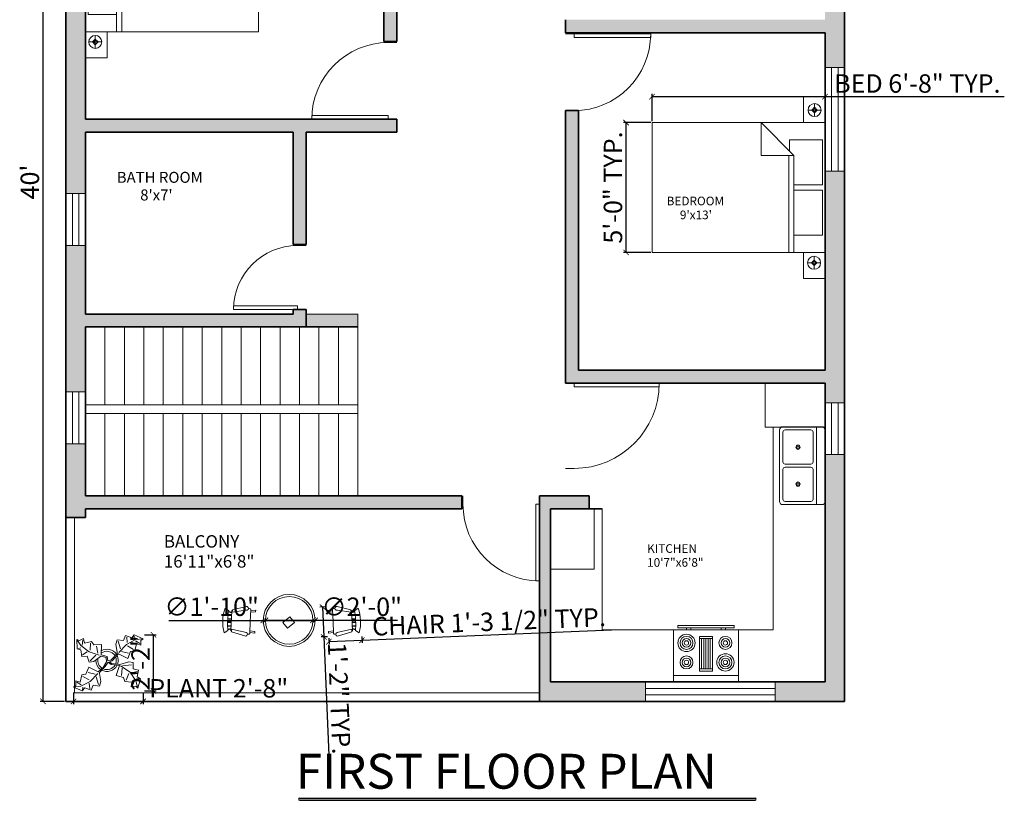
# Model space of a CAD drawing. Units: inches. Extents: x 3799 to 20199, y 1682 to 8087.
# Tile 16 of 30: x 10500 to 10956, y 7270 to 7631. Entities that reach past the tile are written whole.
import ezdxf

# ---------------------------------------------------------------- set-up
doc = ezdxf.new("R2010")
doc.units = ezdxf.units.IN
for name, color, linetype, lineweight in [('A-ANNO-DIMS', 2, 'Continuous', 18), ('A-ANNO-TITL', 7, 'Continuous', 25), ('A-AREA-IDEN', 7, 'Continuous', 18), ('A-DOOR', 3, 'Continuous', 18), ('A-EQPM', 9, 'Continuous', 18), ('A-FLOR-CASE', 32, 'Continuous', 18), ('A-FLOR-FIXT', 9, 'Continuous', 18), ('A-FLOR-RAIL', 217, 'Continuous', 18), ('A-FLOR-STRS', 41, 'Continuous', 18), ('A-FURN', 8, 'Continuous', 18), ('A-GLAZ', 152, 'Continuous', 18), ('A-WALL', 7, 'Continuous', 35), ('A-WALL-PATT', 252, 'Continuous', 13), ('L-PLNT', 94, 'Continuous', 13)]:
    doc.layers.add(name, color=color, linetype=linetype, lineweight=lineweight)
doc.styles.get("Standard").update_dxf_attribs({"font": 'arial.ttf'})
doc.dimstyles.new('ISO-25', dxfattribs={"dimtxt": 8.5, "dimasz": 2.5, "dimexe": 1.25, "dimexo": 0.625, "dimtad": 1, "dimdec": 0, "dimlunit": 3, "dimtxsty": 'Standard', "dimblk": 'ARCHTICK', "dimcen": 2.5, "dimadec": 0, "dimazin": 0, "dimtfac": 1, "dimtdec": 0, "dimtmove": 0, "dimatfit": 3, "dimfxl": 1, "dimarcsym": 0})

# ---------------------------------------------------------------- blocks, each defined once
blk = doc.blocks.new('*U170')
for p, q in [((-900, 0), (-900, 100)), ((0, 0), (0, 100))]:
    blk.add_line(p, q)
blk.add_lwpolyline([(0, 0), (0, -900), (-43.75, -900), (-43.75, 0)], close=True)
blk.add_arc((0, 0), 900, 180, 270)
blk = doc.blocks.new('*U158')
for p, q in [((0, 0), (0, -100)), ((1000, 0), (1000, -100))]:
    blk.add_line(p, q)
blk.add_lwpolyline([(0, 0), (0, 1000), (43.75, 1000), (43.75, 0)], close=True)
blk.add_arc((0, 0), 1000, 0, 90)
blk = doc.blocks.new('*U171')
for p, q in [((-750, 0), (-750, 100)), ((0, 0), (0, 100))]:
    blk.add_line(p, q)
blk.add_lwpolyline([(0, 0), (0, -750), (-43.75, -750), (-43.75, 0)], close=True)
blk.add_arc((0, 0), 750, 180, 270)
blk = doc.blocks.new('*U173')
for p, q in [((0, 0), (0, -100)), ((900, 0), (900, -100))]:
    blk.add_line(p, q)
blk.add_lwpolyline([(0, 0), (0, 900), (43.75, 900), (43.75, 0)], close=True)
blk.add_arc((0, 0), 900, 0, 90)
blk = doc.blocks.new('Bed - Queen')
for p, q in [((0, -80.00003), (0, 0)), ((0, 0), (59.99999, 0)), ((59.99999, 0), (59.99999, -80.00003)), ((7.99999, -1.2), (28.79998, -1.2)), ((7.99999, -14.4), (7.99999, -1.2)), ((28.79998, -1.2), (28.79998, -14.4)), ((31.19999, -1.2), (51.99999, -1.2)), ((31.19999, -14.4), (31.19999, -1.2)), ((51.99999, -1.2), (51.99999, -16.4)), ((0, -14.4), (44.8, -14.4)), ((44.8, -16.8), (0, -16.8)), ((59.99999, -29.6), (44.8, -14.4)), ((44.8, -14.4), (44.8, -29.6)), ((51.99999, -16.4), (46.79936, -16.4)), ((44.8, -29.6), (59.99999, -29.6)), ((59.99999, -80.00003), (0, -80.00003))]:
    blk.add_line(p, q)
blk = doc.blocks.new('Range-Oven - 30 in top')
for p, q in [((0, -3), (30, -3)), ((12, -6), (18, -6)), ((13, -20), (13, -6)), ((14, -6), (14, -20)), ((15, -20), (15, -6)), ((16, -6), (16, -20)), ((17, -20), (17, -6)), ((18, -20), (12, -20)), ((6, -24), (6, -25)), ((8, -25), (8, -24)), ((22, -25), (22, -24)), ((24, -24), (24, -25))]:
    blk.add_line(p, q)
for points in [[(0, -24), (0, 0), (30, 0), (30, -24)], [(12, -21), (12, -5), (18, -5), (18, -21)], [(2, -26), (2, -25), (28, -25), (28, -26)]]:
    blk.add_lwpolyline(points, close=True)
for centre, radius in [((6, -9), 4), ((6, -9), 3), ((6, -9), 2), ((6, -9), 1), ((24, -9), 3), ((24, -9), 2), ((24, -9), 1), ((6, -18), 3), ((6, -18), 2), ((6, -18), 1), ((24, -18), 4), ((24, -18), 3), ((24, -18), 2), ((24, -18), 1)]:
    blk.add_circle(centre, radius)
blk = doc.blocks.new('Sink-double - 36 in top')
for p, q in [((-18, -4), (18, -4)), ((-0.75, -18.5), (-0.75, -6.5)), ((0.75, -6.5), (0.75, -18.5))]:
    blk.add_line(p, q)
for points in [[(-16.5, 0), (16.5, 0)], [(-18, -19.5), (-18, -1.5)], [(18, -1.5), (18, -19.5)], [(-16.5, -18.5), (-16.5, -6.5)], [(-15.5, -5.5), (-1.75, -5.5)], [(1.75, -5.5), (15.5, -5.5)], [(16.5, -6.5), (16.5, -18.5)], [(16.5, -21), (-16.5, -21)], [(-1.75, -19.5), (-15.5, -19.5)], [(15.5, -19.5), (1.75, -19.5)]]:
    blk.add_lwpolyline(points)
for centre, radius in [((-8.5, -12.5), 1), ((-8.5, -12.5), 0.5), ((8.5, -12.5), 1), ((8.5, -12.5), 0.5)]:
    blk.add_circle(centre, radius)
for centre, radius, start, end in [((-16.5, -1.5), 1.5, 90, 180), ((16.5, -1.5), 1.5, 0, 90), ((-15.5, -6.5), 1, 90, 180), ((-1.75, -6.5), 1, 0, 90), ((1.75, -6.5), 1, 90, 180), ((15.5, -6.5), 1, 0, 90), ((-16.5, -19.5), 1.5, 180, 270), ((-15.5, -18.5), 1, 180, 270), ((-1.75, -18.5), 1, 270, 0), ((1.75, -18.5), 1, 180, 270), ((15.5, -18.5), 1, 270, 0), ((16.5, -19.5), 1.5, 270, 0)]:
    blk.add_arc(centre, radius, start, end)
blk = doc.blocks.new('Chair - Rocking')
for p, q in [((-9, -7.5), (-12, -18.49999)), ((-8, -4.5), (-10, -1.5)), ((-7, -7.5), (-9, -7.5)), ((-9, -18.49999), (-7, -7.5)), ((-8.23428, -6.99939), (-8.3093, -7.47958)), ((-8.23041, -7), (8.23915, -7)), ((-7.5, -4.5), (-7, -7)), ((-6.5, -7), (-7.02225, -4.43)), ((-4.5, -7), (-4.96674, -4.19951)), ((-4, -7), (-4.40532, -4.16272)), ((-1.5, -4.05012), (-1.5, -7)), ((-1, -7), (-1, -4.05012)), ((1, -7), (1, -4.04655)), ((1.5, -4.05012), (1.5, -7)), ((4, -7), (4.40187, -4.18694)), ((4.5, -7), (4.96761, -4.19437)), ((6.5, -7), (7, -4.4057)), ((7.5, -4.5), (7, -7)), ((7, -7.5), (9, -7.5)), ((9, -18.49999), (7, -7.5)), ((8, -4.5), (10, -1.5)), ((8.31071, -7.48854), (8.23449, -7.00073)), ((9, -7.5), (12, -18.49999)), ((-10.36644, -20.64523), (-10.5, -21.49999)), ((-9, -22.49999), (-9.5, -26.49999)), ((0, -22.49999), (-9.5, -22.49999)), ((-8, -26.49999), (-7.5, -22.49999)), ((0, -22.49999), (9.5, -22.49999)), ((8, -26.49999), (7.5, -22.49999)), ((9, -22.49999), (9.5, -26.49999)), ((10.5, -21.49999), (10.3575, -20.58798)), ((-9.5, -26.49999), (-8, -26.49999)), ((9.5, -26.49999), (8, -26.49999))]:
    blk.add_line(p, q)
for centre, radius, start, end in [((0, -34.08333), 34.08333, 72.93847, 107.0615), ((0, -68.25004), 64.25, 93.92211, 97.15267), ((0, -68.25004), 64.25, 82.84733, 93.92211), ((-10.5, -18.99999), 1.58114, 161.5651, 18.43495), ((-9.5, -21.49999), 1, 180, 270), ((10.5, -18.99999), 1.58114, 161.5651, 18.43495), ((9.5, -21.49999), 1, 270, 0)]:
    blk.add_arc(centre, radius, start, end)
blk = doc.blocks.new('Lamp - Table')
for p, q in [((-1, 0), (-7, 0)), ((0, 3), (-3, 0)), ((-3, 0), (0, -3)), ((0, 7), (0, 1)), ((3, 0), (0, 3)), ((0, -3), (3, 0)), ((1, 0), (7, 0)), ((0, -1), (0, -7))]:
    blk.add_line(p, q)
for radius in [7, 1]:
    blk.add_circle((0, 0), radius)
blk = doc.blocks.new('Plant - Rubber or Philodendron')
for p, q in [((-16.2005, 11.4774), (-13.9899, 8.1064)), ((-16.2005, 11.4774), (-14.8639, 10.7964)), ((-16.0159, 6.3329), (-16.2005, 11.4774)), ((-14.8639, 10.7964), (-12.6195, 11.8975)), ((-13.3174, 8.325), (-13.0735, 11.0065)), ((-12.6195, 11.8975), (-12.1909, 9.4345)), ((4.6914, 8.8812), (5.3859, 11.2828)), ((5.3859, 11.2828), (8.8871, 10.7908)), ((8.8871, 10.7908), (9.9809, 13.4933)), ((9.9809, 13.4933), (13.3837, 12.301)), ((15.3859, 11.3055), (10.3916, 8.7942)), ((10.5828, 12.6946), (10.8893, 9.7953)), ((13.3837, 12.301), (14.68, 13.9039)), ((14.5816, 13.2037), (14.3848, 11.8033)), ((14.68, 13.9039), (19.3848, 11.8146)), ((15.2875, 10.6053), (17.5907, 9.2105)), ((19.3848, 11.8146), (15.3859, 11.3055)), ((19.3848, 11.8146), (18.1868, 10.9119)), ((18.1868, 10.9119), (18.1925, 8.4119)), ((-14.0069, 5.8704), (-16.0159, 6.3329)), ((-15.3434, 6.5514), (-13.9984, 6.9884)), ((-13.5868, 2.2894), (-14.0069, 5.8704)), ((-13.9899, 8.1064), (-9.5434, 4.7185)), ((-12.1909, 9.4345), (-8.3829, 10.3)), ((-8.8369, 9.409), (-9.0894, 5.6095)), ((-8.3829, 10.3), (-7.0549, 8.501)), ((-7.0549, 8.501), (-3.0284, 8.6941)), ((-4.8529, 4.012), (-5.7184, 7.82)), ((-3.0284, 8.6941), (-3.0709, 3.1041)), ((4.6914, 8.8812), (5.5014, 4.4831)), ((5.9878, 10.4842), (7.1971, 6.3869)), ((10.3916, 8.7942), (6.2847, 4.4028)), ((14.2977, 6.1031), (10.9934, 7.9956)), ((14.8995, 5.3044), (12.7005, 4.8994)), ((15.7909, 9.1065), (14.8995, 5.3044)), ((18.1925, 8.4119), (15.7909, 9.1065)), ((-10.6784, 2.491), (-13.5868, 2.2894)), ((-13.1329, 3.1804), (-10.6614, 4.727)), ((-9.5858, -0.8715), (-10.6784, 2.491)), ((-9.5434, 4.7185), (-4.1917, 2.9888)), ((-9.1318, 0.0195), (-5.9793, 2.9025)), ((-7.1228, -0.443), (-3.5248, 2.2131)), ((-3.5248, 2.2131), (-3.3011, 2.4355)), ((-3.3011, 2.4355), (-0.5306, 1.7947)), ((-3.0709, 3.1041), (0.0797, 2.3163)), ((-0.5306, 1.7947), (-0.2255, -0.5527)), ((-0.5306, 1.7947), (-0.5306, 1.7947)), ((0.0797, 2.3163), (0.4866, -0.031)), ((0.4866, -0.031), (2.1141, 0.2298)), ((2.1141, 0.2298), (5.4346, 3.9146)), ((6.1032, 3.6844), (2.8262, -0.031)), ((5.4346, 3.9146), (5.5014, 4.4831)), ((11.1089, 1.1958), (6.1032, 3.6844)), ((7.7005, 4.8881), (11.5025, 3.9967)), ((12.7005, 4.8994), (11.1089, 1.1958)), ((-11.3237, -7.2629), (-9.7321, -3.5593)), ((-9.7321, -3.5593), (-4.7264, -6.0479)), ((-7.1228, -0.443), (-9.5858, -0.8715)), ((-2.019, -3.6148), (-4.7264, -6.0479)), ((-4.0579, -6.2781), (-0.9375, -3.1608)), ((-2.019, -3.6148), (-0.2255, -0.5527)), ((-0.9375, -3.1608), (0.5883, -0.8135)), ((0.5883, -0.8135), (2.2447, -2.0916)), ((2.8262, -0.031), (1.3003, -0.5527)), ((1.3003, -0.5527), (2.4193, -1.4655)), ((2.2447, -2.0916), (6.7108, -2.6626)), ((2.4193, -1.4655), (6.895, -2.1175)), ((4.943, -7.9659), (6.7108, -2.6626)), ((11.6605, -0.5413), (6.895, -2.1175)), ((12.3677, -6.1981), (7.219, -2.6772)), ((8.125, -4.0768), (7.7715, -7.9659)), ((8.3544, -2.7453), (13.1973, -2.1704)), ((11.6605, -0.5413), (14.1354, -0.8948)), ((14.1354, -0.8948), (14.1354, -4.4304)), ((14.1354, -4.4304), (16.9638, -5.1375)), ((16.9638, -5.1375), (16.2567, -8.673)), ((-14.4141, -11.4699), (-13.5228, -7.6679)), ((-13.5228, -7.6679), (-11.3237, -7.2629)), ((-12.921, -8.4665), (-9.6166, -10.359)), ((-6.3237, -7.2516), (-10.1257, -6.3602)), ((-9.0148, -11.1577), (-4.9047, -6.8122)), ((-4.611, -12.8477), (-5.8203, -8.7504)), ((-4.1246, -6.8466), (-4.0579, -6.2781)), ((-3.3146, -11.2447), (-4.1246, -6.8466)), ((8.8321, -9.0266), (4.943, -7.9659)), ((9.5392, -11.1479), (8.8321, -9.0266)), ((10.2463, -10.4408), (11.6605, -6.9053)), ((15.5496, -10.7943), (12.3677, -6.1981)), ((16.2567, -5.8446), (13.4283, -6.5517)), ((17.3174, -9.7337), (15.9032, -9.7337)), ((16.2567, -8.673), (18.0245, -9.7337)), ((18.0245, -9.7337), (16.6103, -14.6834)), ((-18.008, -14.1781), (-16.8101, -13.2754)), ((-18.008, -14.1781), (-14.0091, -13.669)), ((-13.3032, -16.2674), (-18.008, -14.1781)), ((-16.8157, -10.7754), (-14.4141, -11.4699)), ((-16.8101, -13.2754), (-16.8157, -10.7754)), ((-13.9107, -12.9688), (-16.2139, -11.574)), ((-14.0091, -13.669), (-9.0148, -11.1577)), ((-12.0069, -14.6645), (-13.3032, -16.2674)), ((-13.2048, -15.5672), (-13.008, -14.1668)), ((-8.6042, -15.8568), (-12.0069, -14.6645)), ((-9.206, -15.0581), (-9.5126, -12.1588)), ((-7.5103, -13.1543), (-8.6042, -15.8568)), ((-4.0092, -13.6463), (-7.5103, -13.1543)), ((-3.3146, -11.2447), (-4.0092, -13.6463)), ((13.4283, -11.5015), (9.5392, -11.1479)), ((13.0748, -13.9763), (13.4283, -11.5015)), ((15.5496, -13.6228), (13.0748, -13.9763)), ((14.8425, -10.7943), (13.7819, -13.2692)), ((16.6103, -14.6834), (15.5496, -10.7943)), ((16.6103, -14.6834), (15.5496, -13.6228))]:
    blk.add_line(p, q)
for centre, radius, start, end in [((0, 0), 6.1275, 34.37569, 120.1028), ((0.0308, 0.1664), 6, 178.6147, 235.1169), ((0.0308, 0.1664), 5, 168.1647, 238.6725), ((-0.0601, -0.2075), 5.2461, 33.82192, 124.9414), ((-0.2664, 0.1682), 5.2775, 338.4094, 20.03007), ((-0.098, 0.1364), 6.1288, 341.2017, 26.09184), ((-0.0234, 0.3825), 6.1492, 242.5812, 331.2714), ((-0.1102, 0.4886), 5.2883, 247.3711, 327.472)]:
    blk.add_arc(centre, radius, start, end)
blk = doc.blocks.new('_ArchTick')
at = {"color": 0, "linetype": 'ByBlock', "const_width": 0.15}
blk.add_lwpolyline([(-0.5, -0.5), (0.5, 0.5)], dxfattribs=at)
blk = doc.blocks.new('*D176')
at = {"layer": 'A-ANNO-DIMS', "color": 0, "lineweight": -2, "transparency": 16777216}
for p, q in [((10521.25, 7795.62), (10509.98, 7795.62)), ((10511.23, 7795.62), (10511.23, 7315.62)), ((10521.25, 7315.62), (10509.98, 7315.62))]:
    blk.add_line(p, q, dxfattribs=at)
at = {"layer": 'Defpoints', "color": 0, "transparency": 16777216}
for p in [(10521.87, 7795.62), (10511.23, 7315.62), (10521.87, 7315.62)]:
    blk.add_point(p, dxfattribs=at)
at = {"layer": 'A-ANNO-DIMS', "color": 0, "lineweight": -2, "transparency": 16777216, "xscale": 2.5, "yscale": 2.5, "zscale": 2.5}
for p, rotation in [((10511.23, 7795.62), 90), ((10511.23, 7315.62), 270)]:
    blk.add_blockref('_ArchTick', p, dxfattribs=dict(at, rotation=rotation))
at = {"layer": 'A-ANNO-DIMS', "color": 0, "transparency": 16777216, "insert": (10506.27, 7555.62), "char_height": 8.5, "attachment_point": 5, "rotation": 90}
blk.add_mtext("40'", dxfattribs=at)
blk = doc.blocks.new('WIN-24IN-9IN-FRAME')
for p, q in [((0, 24), (9, 24)), ((3, 0), (3, 24)), ((6, 0), (6, 24)), ((0, 0), (9, 0))]:
    blk.add_line(p, q)
blk = doc.blocks.new('WIN-48IN-9IN-FRAME')
for p, q in [((0, 0), (0, 9)), ((48, 6), (0, 6)), ((48, 0), (48, 9)), ((48, 3), (0, 3))]:
    blk.add_line(p, q)
blk = doc.blocks.new('WIN-60IN-9IN-FRAME')
for p, q in [((0, 9), (0, 0)), ((60, 6), (0, 6)), ((60, 9), (60, 0)), ((60, 3), (0, 3))]:
    blk.add_line(p, q)
blk = doc.blocks.new('*D252')
at = {"layer": 'A-ANNO-DIMS', "color": 0, "lineweight": -2, "transparency": 16777216}
for p, q in [((10792.87, 7583.69), (10792.87, 7596.31)), ((10792.87, 7595.06), (10872.87, 7595.06)), ((10872.87, 7583.69), (10872.87, 7596.31)), ((10872.87, 7595.06), (10955.77, 7595.06))]:
    blk.add_line(p, q, dxfattribs=at)
at = {"layer": 'Defpoints', "color": 0, "transparency": 16777216}
for p in [(10872.87, 7595.06), (10792.87, 7583.06), (10872.87, 7583.06)]:
    blk.add_point(p, dxfattribs=at)
at = {"layer": 'A-ANNO-DIMS', "color": 0, "lineweight": -2, "transparency": 16777216, "xscale": 2.5, "yscale": 2.5, "zscale": 2.5, "rotation": 180}
blk.add_blockref('_ArchTick', (10792.87, 7595.06), dxfattribs=at)
at = {"layer": 'A-ANNO-DIMS', "color": 0, "lineweight": -2, "transparency": 16777216, "xscale": 2.5, "yscale": 2.5, "zscale": 2.5}
blk.add_blockref('_ArchTick', (10872.87, 7595.06), dxfattribs=at)
at = {"layer": 'A-ANNO-DIMS', "color": 0, "transparency": 16777216, "insert": (10915.57, 7600.03), "char_height": 8.5, "attachment_point": 5}
blk.add_mtext('BED 6\'-8" TYP.', dxfattribs=at)
blk = doc.blocks.new('*D253')
at = {"layer": 'A-ANNO-DIMS', "color": 0, "lineweight": -2, "transparency": 16777216}
for p, q in [((10792.25, 7583.06), (10779.62, 7583.06)), ((10780.87, 7523.06), (10780.87, 7583.06)), ((10792.25, 7523.06), (10779.62, 7523.06))]:
    blk.add_line(p, q, dxfattribs=at)
at = {"layer": 'Defpoints', "color": 0, "transparency": 16777216}
for p in [(10780.87, 7583.06), (10792.87, 7583.06), (10792.87, 7523.06)]:
    blk.add_point(p, dxfattribs=at)
at = {"layer": 'A-ANNO-DIMS', "color": 0, "lineweight": -2, "transparency": 16777216, "xscale": 2.5, "yscale": 2.5, "zscale": 2.5}
for p, rotation in [((10780.87, 7583.06), 90), ((10780.87, 7523.06), 270)]:
    blk.add_blockref('_ArchTick', p, dxfattribs=dict(at, rotation=rotation))
at = {"layer": 'A-ANNO-DIMS', "color": 0, "transparency": 16777216, "insert": (10775.91, 7553.06), "char_height": 8.5, "attachment_point": 5, "rotation": 90}
blk.add_mtext('5\'-0" TYP.', dxfattribs=at)
blk = doc.blocks.new('*D318')
at = {"layer": 'A-ANNO-DIMS', "color": 0, "lineweight": -2, "transparency": 16777216}
for p, q in [((10658.76, 7343.85), (10774.17, 7348.63)), ((10643.4, 7344.88), (10643.52, 7341.97)), ((10658.69, 7345.52), (10658.81, 7342.6)), ((10643.47, 7343.22), (10658.76, 7343.85))]:
    blk.add_line(p, q, dxfattribs=at)
at = {"layer": 'Defpoints', "color": 0, "transparency": 16777216}
for p in [(10643.38, 7345.51), (10658.66, 7346.14), (10658.76, 7343.85)]:
    blk.add_point(p, dxfattribs=at)
at = {"layer": 'A-ANNO-DIMS', "color": 0, "lineweight": -2, "transparency": 16777216, "xscale": 2.5, "yscale": 2.5, "zscale": 2.5}
for p, rotation in [((10643.47, 7343.22), 182.3732176474188), ((10658.76, 7343.85), 2.373217647418867)]:
    blk.add_blockref('_ArchTick', p, dxfattribs=dict(at, rotation=rotation))
at = {"layer": 'A-ANNO-DIMS', "color": 0, "transparency": 16777216, "insert": (10717.51, 7351.31), "char_height": 8.5, "attachment_point": 5, "rotation": 2.3732}
blk.add_mtext('CHAIR 1\'-3 1/2" TYP.', dxfattribs=at)
blk = doc.blocks.new('*D319')
at = {"layer": 'A-ANNO-DIMS', "color": 0, "lineweight": -2, "transparency": 16777216}
for p, q in [((10642.18, 7359.32), (10639.26, 7359.2)), ((10640.51, 7359.25), (10641.08, 7345.41)), ((10642.75, 7345.48), (10639.84, 7345.36)), ((10641.08, 7345.41), (10643.35, 7290.7))]:
    blk.add_line(p, q, dxfattribs=at)
at = {"layer": 'Defpoints', "color": 0, "transparency": 16777216}
for p in [(10642.8, 7359.34), (10641.08, 7345.41), (10643.38, 7345.51)]:
    blk.add_point(p, dxfattribs=at)
at = {"layer": 'A-ANNO-DIMS', "color": 0, "lineweight": -2, "transparency": 16777216, "xscale": 2.5, "yscale": 2.5, "zscale": 2.5}
for p, rotation in [((10640.51, 7359.25), 92.37321764741522), ((10641.08, 7345.41), 272.3732176474152)]:
    blk.add_blockref('_ArchTick', p, dxfattribs=dict(at, rotation=rotation))
at = {"layer": 'A-ANNO-DIMS', "color": 0, "transparency": 16777216, "insert": (10647.16, 7317.01), "char_height": 8.5, "attachment_point": 5, "rotation": 272.3732}
blk.add_mtext('1\'-2" TYP.', dxfattribs=at)
blk = doc.blocks.new('*D352')
at = {"layer": 'A-ANNO-DIMS', "color": 0, "lineweight": -2, "transparency": 16777216}
for p, q in [((10525.36, 7319.78), (10525.36, 7314.33)), ((10557.53, 7319.78), (10557.53, 7314.33)), ((10525.36, 7315.58), (10557.53, 7315.58)), ((10557.53, 7315.58), (10625.02, 7315.58))]:
    blk.add_line(p, q, dxfattribs=at)
at = {"layer": 'Defpoints', "color": 0, "transparency": 16777216}
for p in [(10525.36, 7320.41), (10557.53, 7320.41), (10557.53, 7315.58)]:
    blk.add_point(p, dxfattribs=at)
at = {"layer": 'A-ANNO-DIMS', "color": 0, "lineweight": -2, "transparency": 16777216, "xscale": 2.5, "yscale": 2.5, "zscale": 2.5, "rotation": 180}
blk.add_blockref('_ArchTick', (10525.36, 7315.58), dxfattribs=at)
at = {"layer": 'A-ANNO-DIMS', "color": 0, "lineweight": -2, "transparency": 16777216, "xscale": 2.5, "yscale": 2.5, "zscale": 2.5}
blk.add_blockref('_ArchTick', (10557.53, 7315.58), dxfattribs=at)
at = {"layer": 'A-ANNO-DIMS', "color": 0, "transparency": 16777216, "insert": (10592.52, 7320.55), "char_height": 8.5, "attachment_point": 5}
blk.add_mtext('PLANT 2\'-8"', dxfattribs=at)
blk = doc.blocks.new('*D353')
at = {"layer": 'A-ANNO-DIMS', "color": 0, "lineweight": -2, "transparency": 16777216}
for p, q in [((10558.15, 7346.36), (10563.6, 7346.36)), ((10562.35, 7320.41), (10562.35, 7346.36)), ((10558.15, 7320.41), (10563.6, 7320.41))]:
    blk.add_line(p, q, dxfattribs=at)
at = {"layer": 'Defpoints', "color": 0, "transparency": 16777216}
for p in [(10557.53, 7346.36), (10562.35, 7346.36), (10557.53, 7320.41)]:
    blk.add_point(p, dxfattribs=at)
at = {"layer": 'A-ANNO-DIMS', "color": 0, "lineweight": -2, "transparency": 16777216, "xscale": 2.5, "yscale": 2.5, "zscale": 2.5}
for p, rotation in [((10562.35, 7346.36), 90), ((10562.35, 7320.41), 270)]:
    blk.add_blockref('_ArchTick', p, dxfattribs=dict(at, rotation=rotation))
at = {"layer": 'A-ANNO-DIMS', "color": 0, "transparency": 16777216, "insert": (10557.46, 7333.38), "char_height": 8.5, "attachment_point": 5, "rotation": 90}
blk.add_mtext('2\'-2"', dxfattribs=at)
blk = doc.blocks.new('*D391')
at = {"layer": 'A-ANNO-DIMS', "color": 0, "lineweight": -2, "transparency": 16777216}
for p in [(10613.1, 7353.04), (10675.19, 7353.04)]:
    blk.add_line(p, (10637.1, 7353.04), dxfattribs=at)
at = {"layer": 'Defpoints', "color": 0, "transparency": 16777216}
for p in [(10613.1, 7353.04), (10637.1, 7353.04)]:
    blk.add_point(p, dxfattribs=at)
at = {"layer": 'A-ANNO-DIMS', "color": 0, "lineweight": -2, "transparency": 16777216, "xscale": 2.5, "yscale": 2.5, "zscale": 2.5}
for p, rotation in [((10613.1, 7353.04), 359.9981044646316), ((10637.1, 7353.04), 179.9981044646316)]:
    blk.add_blockref('_ArchTick', p, dxfattribs=dict(at, rotation=rotation))
at = {"layer": 'A-ANNO-DIMS', "color": 0, "transparency": 16777216, "insert": (10658.65, 7358.24), "char_height": 8.5, "attachment_point": 5, "rotation": 359.9981}
blk.add_mtext('∅2\'-0"', dxfattribs=at)
blk = doc.blocks.new('*D392')
at = {"layer": 'A-ANNO-DIMS', "color": 0, "lineweight": -2, "transparency": 16777216}
for p in [(10569.4, 7353.04), (10636.1, 7353.04)]:
    blk.add_line(p, (10614.1, 7353.04), dxfattribs=at)
at = {"layer": 'Defpoints', "color": 0, "transparency": 16777216}
for p in [(10614.1, 7353.04), (10636.1, 7353.04)]:
    blk.add_point(p, dxfattribs=at)
at = {"layer": 'A-ANNO-DIMS', "color": 0, "lineweight": -2, "transparency": 16777216, "xscale": 2.5, "yscale": 2.5, "zscale": 2.5}
for p, rotation in [((10614.1, 7353.04), 0.0020678567677366), ((10636.1, 7353.04), 180.0020678567677)]:
    blk.add_blockref('_ArchTick', p, dxfattribs=dict(at, rotation=rotation))
at = {"layer": 'A-ANNO-DIMS', "color": 0, "transparency": 16777216, "insert": (10589.25, 7358.24), "char_height": 8.5, "attachment_point": 5, "rotation": 0.0021}
blk.add_mtext('∅1\'-10"', dxfattribs=at)

msp = doc.modelspace()

# ---------------------------------------------------------------- hatches: boundary and pattern name
at = {"layer": 'A-ANNO-TITL'}
h = msp.add_hatch(color=256, dxfattribs=at)
h.dxf.hatch_style = 1
h.paths.add_polyline_path([(10840.51, 7270.89), (10629.95, 7270.89, 1), (10629.95, 7269.89), (10840.51, 7269.89, 1)])
at = {"layer": 'A-WALL-PATT'}
h = msp.add_hatch(color=256, dxfattribs=at)
h.dxf.hatch_style = 1
h.paths.add_polyline_path([(10588.75, 7795.62), (10521.87, 7795.62), (10521.87, 7685.33), (10530.87, 7685.33), (10530.87, 7696.98), (10530.87, 7710.62), (10620.87, 7710.62), (10620.87, 7716.62), (10530.87, 7716.62), (10530.87, 7786.62), (10588.75, 7786.62)])
h.paths.add_polyline_path([(10682.68, 7795.62), (10612.75, 7795.62), (10612.75, 7786.62), (10650.87, 7786.62), (10650.87, 7716.62), (10650.87, 7710.62), (10668.87, 7710.62), (10668.87, 7620.62), (10674.87, 7620.62), (10674.87, 7710.62), (10752.87, 7710.62), (10752.87, 7666.62), (10758.87, 7666.62), (10758.87, 7756.62), (10752.87, 7756.62), (10752.87, 7716.62), (10656.87, 7716.62), (10656.87, 7786.62), (10682.68, 7786.62)])
h.paths.add_polyline_path([(10881.87, 7795.62), (10706.68, 7795.62), (10706.68, 7786.62), (10752.87, 7786.62), (10758.87, 7786.62), (10872.87, 7786.62), (10872.87, 7747.36), (10881.87, 7747.36)])
h.paths.add_polyline_path([(10881.87, 7699.36), (10872.87, 7699.36), (10872.87, 7630.62), (10752.87, 7630.62), (10752.87, 7624.62), (10872.87, 7624.62), (10872.87, 7608.58), (10881.87, 7608.58)])
h.paths.add_polyline_path([(10674.87, 7584.62), (10530.87, 7584.62), (10530.87, 7637.33), (10521.87, 7637.33), (10521.87, 7550.27), (10530.87, 7550.27), (10530.87, 7578.62), (10626.87, 7578.62), (10626.87, 7526.73), (10632.87, 7526.73), (10632.87, 7578.62), (10674.87, 7578.62)])
h.paths.add_polyline_path([(10530.87, 7488.62), (10632.87, 7488.62), (10632.87, 7496.73), (10628.93, 7496.73), (10626.87, 7496.73), (10626.87, 7494.62), (10530.87, 7494.62), (10530.87, 7526.27), (10521.87, 7526.27), (10521.87, 7458.64), (10530.87, 7458.64)])
h.paths.add_polyline_path([(10656.87, 7494.62), (10632.87, 7494.62), (10632.87, 7488.62), (10656.87, 7488.62)])
h.paths.add_polyline_path([(10530.87, 7434.64), (10521.87, 7434.64), (10521.87, 7400.54), (10530.87, 7400.54), (10530.87, 7404.62), (10704.87, 7404.62), (10704.87, 7410.62), (10530.87, 7410.62)])
h.paths.add_polyline_path([(10745.87, 7404.62), (10763.75, 7404.62), (10763.75, 7410.62), (10740.87, 7410.62), (10740.87, 7315.62), (10789.88, 7315.62), (10789.88, 7324.62), (10745.87, 7324.62)])
h.paths.add_polyline_path([(10881.87, 7429.64), (10872.87, 7429.64), (10872.87, 7408.03), (10872.87, 7324.62), (10849.88, 7324.62), (10849.88, 7315.62), (10881.87, 7315.62)])
h.paths.add_polyline_path([(10881.87, 7560.58), (10872.87, 7560.58), (10872.87, 7468.62), (10758.87, 7468.62), (10758.87, 7588.62), (10752.87, 7588.62), (10752.87, 7462.62), (10872.87, 7462.62), (10872.87, 7453.64), (10881.87, 7453.64)])

# ---------------------------------------------------------------- linework, layer by layer
at = {"layer": 'A-ANNO-TITL'}
for p, q in [((10629.95, 7270.89), (10840.51, 7270.89)), ((10629.95, 7269.89), (10840.51, 7269.89))]:
    msp.add_line(p, q, dxfattribs=at)
for centre, start, end in [((10629.95, 7270.39), 90, 270), ((10840.51, 7270.39), 270, 90)]:
    msp.add_arc(centre, 0.5, start, end, dxfattribs=at)
at = {"layer": 'A-FLOR-CASE'}
for p, q in [((10845.14, 7442.32), (10845.14, 7462.62)), ((10848.87, 7442.32), (10845.14, 7442.32)), ((10848.87, 7348.62), (10848.87, 7442.32)), ((10848.87, 7442.32), (10872.87, 7442.32)), ((10769.87, 7348.62), (10769.87, 7404.62)), ((10769.87, 7348.62), (10848.87, 7348.62))]:
    msp.add_line(p, q, dxfattribs=at)
at = {"layer": 'A-FLOR-RAIL'}
for q in [(10525.8, 7400.54), (10740.87, 7319.62)]:
    msp.add_line((10525.8, 7319.62), q, dxfattribs=at)
at = {"layer": 'A-FLOR-STRS'}
for p, q in [((10632.87, 7494.62), (10656.87, 7494.62)), ((10656.87, 7488.62), (10656.87, 7494.62)), ((10539.87, 7488.62), (10539.87, 7452.62)), ((10548.87, 7488.62), (10548.87, 7452.62)), ((10557.87, 7488.62), (10557.87, 7452.62)), ((10566.87, 7488.62), (10566.87, 7452.62)), ((10575.87, 7488.62), (10575.87, 7452.62)), ((10584.87, 7488.62), (10584.87, 7452.62)), ((10593.87, 7488.62), (10593.87, 7452.62)), ((10602.87, 7488.62), (10602.87, 7452.62)), ((10611.87, 7488.62), (10611.87, 7452.62)), ((10620.87, 7488.62), (10620.87, 7452.62)), ((10629.87, 7488.62), (10629.87, 7452.62)), ((10638.87, 7488.62), (10638.87, 7452.62)), ((10647.87, 7488.62), (10647.87, 7452.62)), ((10656.87, 7488.62), (10656.87, 7410.62)), ((10656.87, 7452.62), (10530.87, 7452.62)), ((10656.87, 7448.62), (10530.87, 7448.62)), ((10539.87, 7448.62), (10539.87, 7410.62)), ((10548.87, 7448.62), (10548.87, 7410.62)), ((10557.87, 7448.62), (10557.87, 7410.62)), ((10566.87, 7448.62), (10566.87, 7410.62)), ((10575.87, 7448.62), (10575.87, 7410.62)), ((10584.87, 7448.62), (10584.87, 7410.62)), ((10593.87, 7448.62), (10593.87, 7410.62)), ((10602.87, 7448.62), (10602.87, 7410.62)), ((10611.87, 7448.62), (10611.87, 7410.62)), ((10620.87, 7448.62), (10620.87, 7410.62)), ((10629.87, 7448.62), (10629.87, 7410.62)), ((10638.87, 7448.62), (10638.87, 7410.62)), ((10647.87, 7448.62), (10647.87, 7410.62))]:
    msp.add_line(p, q, dxfattribs=at)
at = {"layer": 'A-FURN'}
for points in [[(10530.87, 7624.98), (10540.87, 7624.98), (10540.87, 7612.98), (10530.87, 7612.98)], [(10872.87, 7583.06), (10862.87, 7583.06), (10862.87, 7595.06), (10872.87, 7595.06)], [(10872.87, 7523.06), (10862.87, 7523.06), (10862.87, 7511.06), (10872.87, 7511.06)], [(10745.87, 7404.62), (10766.06, 7404.62), (10766.06, 7376.7), (10745.87, 7376.7)], [(10622.13, 7352.05), (10625.4, 7354.75), (10627.6, 7352.09), (10624.33, 7349.4)]]:
    msp.add_lwpolyline(points, close=True, dxfattribs=at)
for radius in [12, 11]:
    msp.add_circle((10625.1, 7353.04), radius, dxfattribs=at)
at = {"layer": 'A-WALL'}
for p, q in [((10521.87, 7795.62), (10521.87, 7315.62)), ((10881.87, 7315.62), (10881.87, 7795.62)), ((10530.87, 7710.62), (10530.87, 7584.62)), ((10668.87, 7710.62), (10668.87, 7620.62)), ((10674.87, 7710.62), (10674.87, 7620.62)), ((10752.87, 7630.62), (10752.87, 7624.62)), ((10872.87, 7624.62), (10752.87, 7624.62)), ((10872.87, 7468.62), (10872.87, 7624.62)), ((10674.87, 7620.62), (10668.87, 7620.62)), ((10758.87, 7588.62), (10752.87, 7588.62)), ((10752.87, 7588.62), (10752.87, 7462.62)), ((10758.87, 7588.62), (10758.87, 7468.62)), ((10674.87, 7584.62), (10530.87, 7584.62)), ((10674.87, 7584.62), (10674.87, 7578.62)), ((10530.87, 7578.62), (10530.87, 7494.62)), ((10626.87, 7578.62), (10530.87, 7578.62)), ((10626.87, 7578.62), (10626.87, 7526.73)), ((10674.87, 7578.62), (10632.87, 7578.62)), ((10632.87, 7578.62), (10632.87, 7526.73)), ((10626.87, 7526.73), (10632.87, 7526.73)), ((10626.87, 7494.62), (10530.87, 7494.62)), ((10626.87, 7496.73), (10632.87, 7496.73)), ((10626.87, 7496.73), (10626.87, 7494.62)), ((10632.87, 7496.73), (10632.87, 7488.62)), ((10656.87, 7488.62), (10530.87, 7488.62)), ((10530.87, 7488.62), (10530.87, 7410.62)), ((10872.87, 7468.62), (10758.87, 7468.62)), ((10872.87, 7462.62), (10752.87, 7462.62)), ((10872.87, 7324.62), (10872.87, 7462.62)), ((10530.87, 7410.62), (10704.87, 7410.62)), ((10704.87, 7404.62), (10704.87, 7410.62)), ((10740.87, 7315.62), (10740.87, 7410.62)), ((10740.87, 7410.62), (10763.75, 7410.62)), ((10763.75, 7410.62), (10763.75, 7404.62)), ((10530.87, 7404.62), (10704.87, 7404.62)), ((10530.87, 7404.62), (10530.87, 7400.54)), ((10745.87, 7324.62), (10745.87, 7404.62)), ((10745.87, 7404.62), (10763.75, 7404.62)), ((10763.75, 7404.62), (10769.87, 7404.62)), ((10530.87, 7400.54), (10521.87, 7400.54)), ((10745.87, 7324.62), (10872.87, 7324.62)), ((10521.87, 7315.62), (10881.87, 7315.62))]:
    msp.add_line(p, q, dxfattribs=at)

# ---------------------------------------------------------------- block references
at = {"layer": 'A-DOOR', "xscale": 0.0393700787401575, "yscale": 0.0393700787401575, "zscale": 0.0393700787401575, "rotation": 270}
for name, p in [('*U173', (10756.81, 7624.05)), ('*U170', (10670.93, 7584.62)), ('*U171', (10628.93, 7496.73)), ('*U158', (10756.81, 7462.62))]:
    msp.add_blockref(name, p, dxfattribs=at)
at = {"layer": 'A-DOOR', "xscale": 0.0393700787401575, "yscale": 0.0393700787401575, "zscale": 0.0393700787401575}
msp.add_blockref('*U170', (10740.87, 7406.68), dxfattribs=at)
at = {"layer": 'A-EQPM', "rotation": 180}
msp.add_blockref('Range-Oven - 30 in top', (10832.81, 7324.62), dxfattribs=at)
at = {"layer": 'A-FLOR-FIXT', "rotation": 270}
msp.add_blockref('Sink-double - 36 in top', (10872.87, 7424.53), dxfattribs=at)
at = {"layer": 'A-FURN', "rotation": 90}
msp.add_blockref('Bed - Queen', (10530.87, 7624.98), dxfattribs=at)
at = {"layer": 'A-FURN', "xscale": 0.4285713367347382, "yscale": 0.4285713367347382, "zscale": 0.4285713367347382}
for p in [(10535.42, 7620.34), (10868.02, 7588.86), (10867.83, 7518.27)]:
    msp.add_blockref('Lamp - Table', p, dxfattribs=at)
at = {"layer": 'A-FURN', "xscale": -1, "rotation": 270}
msp.add_blockref('Bed - Queen', (10872.87, 7523.06), dxfattribs=at)
at = {"layer": 'A-FURN', "yscale": 0.5666210211197394, "zscale": 0.5666210211197394}
for p, xscale, rotation in [((10594.37, 7353.05), -0.5666210211197394, 87.6267823525822), ((10658.09, 7353.05), 0.5666210211197394, 272.3732176474178)]:
    msp.add_blockref('Chair - Rocking', p, dxfattribs=dict(at, xscale=xscale, rotation=rotation))
at = {"layer": 'A-GLAZ', "rotation": 90}
msp.add_blockref('WIN-48IN-9IN-FRAME', (10881.87, 7560.58), dxfattribs=at)
at = {"layer": 'A-GLAZ'}
for name, p in [('WIN-24IN-9IN-FRAME', (10521.87, 7526.27)), ('WIN-24IN-9IN-FRAME', (10521.87, 7434.64)), ('WIN-24IN-9IN-FRAME', (10872.87, 7429.64)), ('WIN-60IN-9IN-FRAME', (10789.88, 7315.62))]:
    msp.add_blockref(name, p, dxfattribs=at)
at = {"layer": 'L-PLNT', "xscale": 0.8600817149953272, "yscale": 0.8600817149953272, "zscale": 0.8600817149953272}
msp.add_blockref('Plant - Rubber or Philodendron', (10540.85, 7334.4), dxfattribs=at)

# ---------------------------------------------------------------- texts
at = {"layer": 'A-ANNO-TITL'}
msp.add_text('FIRST FLOOR PLAN', height=16.1299, rotation=0.0011, dxfattribs=at).set_placement((10628.19, 7275.24))
at = {"layer": 'A-AREA-IDEN'}
for s, height, p in [('BATH ROOM', 5.074, (10545.35, 7555.24)), ("       8'x7'", 5.0737, (10545.35, 7547.09)), ('BEDROOM', 4, (10799.64, 7544.85)), ("     9'x13'", 4, (10799.64, 7538.42)), ('BALCONY', 5.76, (10567.12, 7386.66)), ('KITCHEN', 4, (10790.6, 7384.24)), ('16\'11"x6\'8"', 5.7598, (10567.12, 7377.41)), ('10\'7"x6\'8"', 4, (10790.6, 7377.82))]:
    msp.add_text(s, height=height, rotation=0.0008, dxfattribs=at).set_placement(p)

# ---------------------------------------------------------------- dimensions: what is measured, and where the dimension line sits
at = {"layer": 'A-ANNO-DIMS'}
for base, p1, p2, override, picture, middle in [((10511.23, 7315.62), (10521.87, 7795.62), (10521.87, 7315.62), {"dimclrd": 0, "dimclre": 0, "dimclrt": 0}, '*D176', (10506.27, 7555.62)), ((10562.35, 7346.3558), (10557.5259, 7320.406), (10557.5259, 7346.3558), {"dimdec": 1, "dimlfac": 1, "dimrnd": 0, "dimzin": 1, "dimdsep": 46, "dimlunit": 4, "dimfrac": 2}, '*D353', (10557.4576, 7333.3809))]:
    dim = msp.add_linear_dim(base=base, p1=p1, p2=p2, angle=90, dimstyle='ISO-25', override=override, dxfattribs=at)
    dim.commit()
    dim.dimension.update_dxf_attribs({"geometry": picture, "text_midpoint": middle})
for base, p1, p2, text, picture, middle in [((10872.87, 7595.06), (10792.87, 7583.06), (10872.87, 7583.06), 'BED <> TYP.', '*D252', (10915.57, 7600.03)), ((10557.53, 7315.58), (10525.36, 7320.41), (10557.53, 7320.41), 'PLANT <>', '*D352', (10592.52, 7320.55))]:
    dim = msp.add_linear_dim(base=base, p1=p1, p2=p2, text=text, dimstyle='ISO-25', override={"dimdec": 1, "dimlfac": 1, "dimrnd": 0, "dimzin": 1, "dimdsep": 46, "dimlunit": 4, "dimfrac": 2}, dxfattribs=at)
    dim.commit()
    dim.dimension.update_dxf_attribs({"geometry": picture, "text_midpoint": middle})
for base, p1, p2, angle, text, picture, middle in [((10780.87, 7583.06), (10792.87, 7523.06), (10792.87, 7583.06), 90, '<> TYP.', '*D253', (10775.91, 7553.06)), ((10658.76, 7343.85), (10643.38, 7345.51), (10658.66, 7346.14), 2.3732, 'CHAIR <> TYP.', '*D318', (10717.51, 7351.31)), ((10641.08, 7345.41), (10642.8, 7359.34), (10643.38, 7345.51), 272.3732, '<> TYP.', '*D319', (10647.16, 7317.01))]:
    dim = msp.add_linear_dim(base=base, p1=p1, p2=p2, angle=angle, text=text, dimstyle='ISO-25', override={"dimdec": 1, "dimlfac": 1, "dimrnd": 0, "dimzin": 1, "dimdsep": 46, "dimlunit": 4, "dimfrac": 2}, dxfattribs=at)
    dim.commit()
    dim.dimension.update_dxf_attribs({"geometry": picture, "text_midpoint": middle})
for p1, p2, picture, middle in [((10636.1, 7353.04), (10614.1, 7353.04), '*D392', (10589.25, 7353.04)), ((10613.1, 7353.04), (10637.1, 7353.04), '*D391', (10658.65, 7353.04))]:
    dim = msp.add_diameter_dim_2p(p1=p1, p2=p2, dimstyle='ISO-25', override={"dimdec": 1, "dimlfac": 1, "dimrnd": 0, "dimzin": 1, "dimdsep": 46, "dimlunit": 4, "dimfrac": 2}, dxfattribs=at)
    dim.commit()
    dim.dimension.update_dxf_attribs({"geometry": picture, "text_midpoint": middle, "dimtype": 163})

doc.saveas('drawing.dxf')
